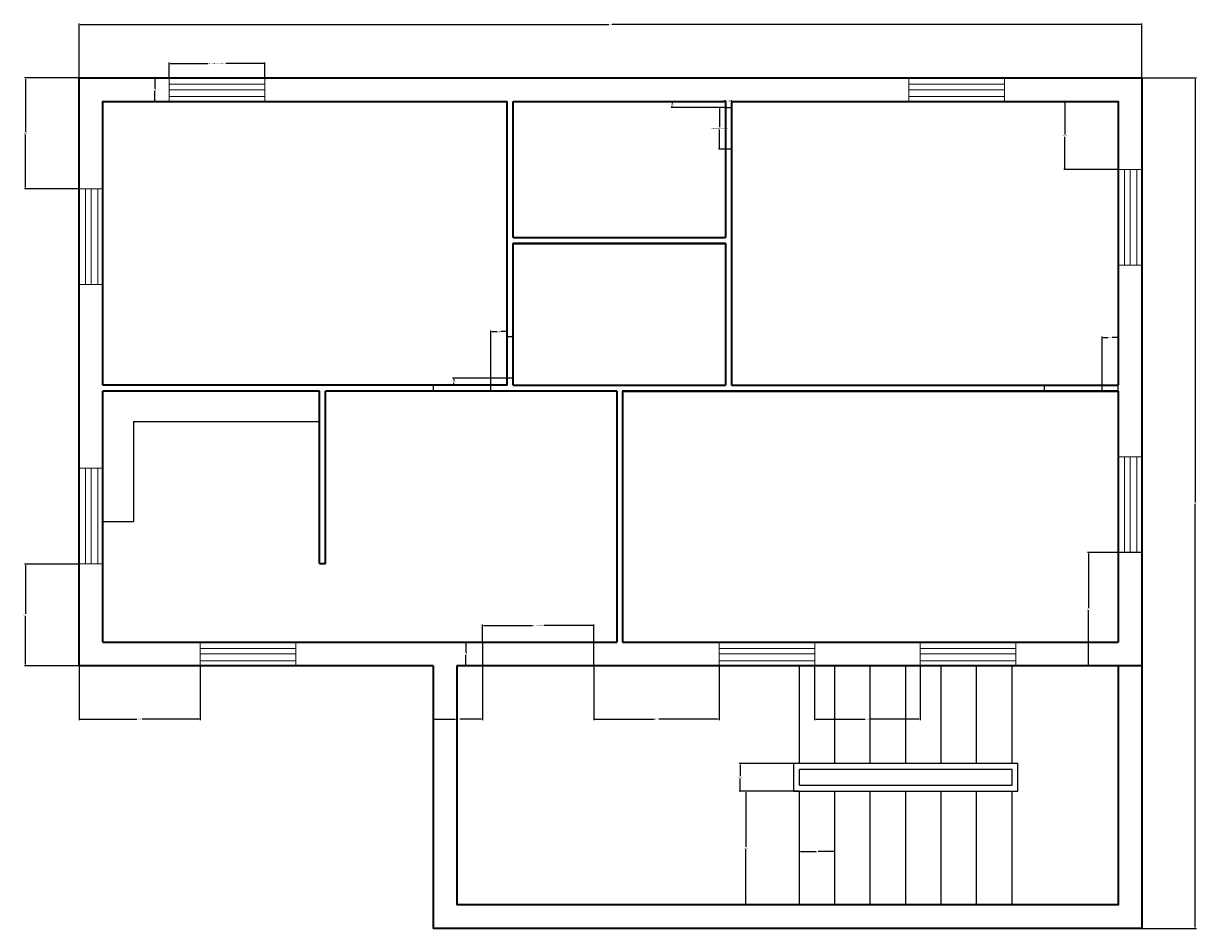
# Model space of a CAD drawing. Units: feet. Extents: x 1914 to 2338, y 2098 to 2528.
# Tile 2 of 3: x 2140 to 2338, y 2107 to 2260. Entities that reach past the tile are written whole.
import ezdxf

# ---------------------------------------------------------------- set-up
doc = ezdxf.new("R2010")
doc.units = ezdxf.units.FT
for name, color, linetype, lineweight in [('A-ANNO-DIMS', 2, 'Continuous', 18), ('A-DOOR', 3, 'Continuous', 25), ('A-FLOR-CASE', 8, 'Continuous', 25), ('A-FLOR-STRS', 7, 'Continuous', 25), ('A-GLAZ', 4, 'Continuous', 18), ('A-WALL', 7, 'Continuous', 35)]:
    doc.layers.add(name, color=color, linetype=linetype, lineweight=lineweight)
doc.styles.get("Standard").update_dxf_attribs({"font": 'arial.ttf'})
doc.dimstyles.get("Standard").update_dxf_attribs({"dimtxt": 0.18, "dimasz": 0.18, "dimexe": 0.18, "dimexo": 0.0625, "dimgap": 0.09, "dimtad": 0, "dimtih": 1, "dimtoh": 1, "dimdec": 1, "dimzin": 0, "dimdsep": 46, "dimlunit": 3, "dimtxsty": 'Standard', "dimcen": 0.09, "dimadec": 0, "dimazin": 0, "dimtfac": 1, "dimtdec": 1, "dimtofl": 0, "dimtmove": 0, "dimatfit": 3, "dimfxl": 1, "dimtolj": 1, "dimtzin": 0, "dimarcsym": 0})

# ---------------------------------------------------------------- blocks, each defined once
blk = doc.blocks.new('WIN-PLAN')
for p, q in [((0, 0), (0, 4)), ((16.2, 4), (16.2, 0)), ((16.2, 2.93), (0, 2.93)), ((16.2, 1.98), (0, 1.98)), ((16.2, 0.84), (0, 0.84))]:
    blk.add_line(p, q)
blk = doc.blocks.new('WIN-PLAN-OUTER-EDGE')
for p, q in [((0, 0), (0, 4)), ((0, 4), (16.2, 4)), ((16.2, 4), (16.2, 0)), ((16.2, 2.93), (0, 2.93)), ((16.2, 1.98), (0, 1.98)), ((16.2, 0.84), (0, 0.84))]:
    blk.add_line(p, q)
blk.add_lwpolyline([(0, 4), (16.2, 4)])
blk = doc.blocks.new('STAIR-RETURN-FLIGHT')
for p, q in [((1, 23.92), (1, 40.5)), ((7, 23.92), (7, 40.5)), ((13, 23.92), (13, 40.5)), ((19, 23.92), (19, 40.5)), ((25, 23.92), (25, 40.5)), ((31, 23.92), (31, 40.5)), ((37, 23.92), (37, 40.5)), ((1, 20.25), (1, 22.92)), ((37, 20.25), (37, 22.92)), ((1, 0), (1, 19.25)), ((7, 0), (7, 19.25)), ((13, 0), (13, 19.25)), ((19, 0), (19, 19.25)), ((25, 0), (25, 19.25)), ((31, 0), (31, 19.25)), ((37, 0), (37, 19.25))]:
    blk.add_line(p, q)
blk.add_lwpolyline([(0, 19.25), (38, 19.25), (38, 23.92), (0, 23.92)], close=True)
for points in [[(37, 22.92), (1, 22.92)], [(1, 20.25), (37, 20.25)]]:
    blk.add_lwpolyline(points)
blk = doc.blocks.new('COUNTER-L')
for p, q in [((5.19, 16.93), (5.19, 0)), ((5.19, 16.93), (36.73, 16.93)), ((0, 0), (5.19, 0))]:
    blk.add_line(p, q)
blk = doc.blocks.new('OPENING-ENTRY')
for points in [[(0, 4), (0, 0)], [(18.83, 0), (18.83, 4)]]:
    blk.add_lwpolyline(points)
blk = doc.blocks.new('OPENING-INTERIOR-WIDE')
blk.add_lwpolyline([(9.8, 0), (9.8, 1), (0, 1), (0, 0)], close=True)
blk = doc.blocks.new('OPENING-INTERIOR-NARROW')
blk.add_lwpolyline([(0, 7.05), (1, 7.05), (1, 0), (0, 0)], close=True)
blk = doc.blocks.new('*D10')
at = {"layer": 'A-ANNO-DIMS', "color": 0, "lineweight": -2, "transparency": 16777216}
for p, q in [((2164.45, 2250.91), (2164.45, 2253.46)), ((2164.63, 2253.28), (2171.05, 2253.28)), ((2180.47, 2253.28), (2174.05, 2253.28)), ((2180.65, 2250.91), (2180.65, 2253.46))]:
    blk.add_line(p, q, dxfattribs=at)
at = {"layer": 'A-ANNO-DIMS', "color": 0, "transparency": 16777216}
for points in [[(2164.63, 2253.31), (2164.63, 2253.25), (2164.45, 2253.28)], [(2180.47, 2253.31), (2180.47, 2253.25), (2180.65, 2253.28)]]:
    blk.add_solid(points, dxfattribs=at)
at = {"layer": 'Defpoints', "color": 0, "transparency": 16777216}
for p in [(2180.65, 2253.28), (2164.45, 2250.85), (2180.65, 2250.85)]:
    blk.add_point(p, dxfattribs=at)
at = {"layer": 'A-ANNO-DIMS', "color": 0, "transparency": 16777216, "insert": (2172.55, 2253.28), "char_height": 0.18, "attachment_point": 5}
blk.add_mtext('\\A1;EDGE WINDOW 16 TYP.', dxfattribs=at)
blk = doc.blocks.new('*D11')
at = {"layer": 'A-ANNO-DIMS', "color": 0, "lineweight": -2, "transparency": 16777216}
for p, q in [((2164.39, 2250.85), (2161.84, 2250.85)), ((2162.02, 2250.67), (2162.02, 2249.03)), ((2162.02, 2247.03), (2162.02, 2248.67)), ((2164.39, 2246.85), (2161.84, 2246.85))]:
    blk.add_line(p, q, dxfattribs=at)
at = {"layer": 'A-ANNO-DIMS', "color": 0, "transparency": 16777216}
for points in [[(2161.99, 2250.67), (2162.05, 2250.67), (2162.02, 2250.85)], [(2161.99, 2247.03), (2162.05, 2247.03), (2162.02, 2246.85)]]:
    blk.add_solid(points, dxfattribs=at)
at = {"layer": 'Defpoints', "color": 0, "transparency": 16777216}
for p in [(2162.02, 2250.85), (2164.45, 2250.85), (2164.45, 2246.85)]:
    blk.add_point(p, dxfattribs=at)
at = {"layer": 'A-ANNO-DIMS', "color": 0, "transparency": 16777216, "insert": (2162.02, 2248.85), "char_height": 0.18, "attachment_point": 5}
blk.add_mtext('\\A1;4 TYP.', dxfattribs=at)
blk = doc.blocks.new('*D14')
at = {"layer": 'A-ANNO-DIMS', "color": 0, "lineweight": -2, "transparency": 16777216}
for p, q in [((2258.63, 2245.84), (2257.46, 2245.84)), ((2257.64, 2245.66), (2257.64, 2242.5)), ((2257.64, 2238.97), (2257.64, 2242.13)), ((2258.63, 2238.79), (2257.46, 2238.79))]:
    blk.add_line(p, q, dxfattribs=at)
at = {"layer": 'A-ANNO-DIMS', "color": 0, "transparency": 16777216}
for points in [[(2257.61, 2245.66), (2257.67, 2245.66), (2257.64, 2245.84)], [(2257.61, 2238.97), (2257.67, 2238.97), (2257.64, 2238.79)]]:
    blk.add_solid(points, dxfattribs=at)
at = {"layer": 'Defpoints', "color": 0, "transparency": 16777216}
for p in [(2257.64, 2245.84), (2258.69, 2245.84), (2258.69, 2238.79)]:
    blk.add_point(p, dxfattribs=at)
at = {"layer": 'A-ANNO-DIMS', "color": 0, "transparency": 16777216, "insert": (2257.64, 2242.31), "char_height": 0.18, "attachment_point": 5}
blk.add_mtext('\\A1;NARROW OPENING 7 TYP.', dxfattribs=at)
blk = doc.blocks.new('*D15')
at = {"layer": 'A-ANNO-DIMS', "color": 0, "lineweight": -2, "transparency": 16777216}
for p, q in [((2258.69, 2245.9), (2258.69, 2247.08)), ((2259.69, 2245.9), (2259.69, 2247.08)), ((2258.51, 2246.9), (2258.33, 2246.9)), ((2259.87, 2246.9), (2260.05, 2246.9))]:
    blk.add_line(p, q, dxfattribs=at)
at = {"layer": 'A-ANNO-DIMS', "color": 0, "transparency": 16777216}
for points in [[(2258.51, 2246.93), (2258.51, 2246.87), (2258.69, 2246.9)], [(2259.87, 2246.93), (2259.87, 2246.87), (2259.69, 2246.9)]]:
    blk.add_solid(points, dxfattribs=at)
at = {"layer": 'Defpoints', "color": 0, "transparency": 16777216}
for p in [(2258.69, 2245.84), (2259.69, 2246.9), (2259.69, 2245.84)]:
    blk.add_point(p, dxfattribs=at)
at = {"layer": 'A-ANNO-DIMS', "color": 0, "transparency": 16777216, "insert": (2259.19, 2246.9), "char_height": 0.18, "attachment_point": 5}
blk.add_mtext('\\A1;1 TYP.', dxfattribs=at)
blk = doc.blocks.new('*D16')
at = {"layer": 'A-ANNO-DIMS', "color": 0, "lineweight": -2, "transparency": 16777216}
for p, q in [((2217.53, 2155.41), (2217.53, 2158.35)), ((2217.71, 2158.17), (2225.96, 2158.17)), ((2236.18, 2158.17), (2227.93, 2158.17)), ((2236.36, 2155.41), (2236.36, 2158.35))]:
    blk.add_line(p, q, dxfattribs=at)
at = {"layer": 'A-ANNO-DIMS', "color": 0, "transparency": 16777216}
for points in [[(2217.71, 2158.2), (2217.71, 2158.14), (2217.53, 2158.17)], [(2236.18, 2158.2), (2236.18, 2158.14), (2236.36, 2158.17)]]:
    blk.add_solid(points, dxfattribs=at)
at = {"layer": 'Defpoints', "color": 0, "transparency": 16777216}
for p in [(2236.36, 2158.17), (2217.53, 2155.35), (2236.36, 2155.35)]:
    blk.add_point(p, dxfattribs=at)
at = {"layer": 'A-ANNO-DIMS', "color": 0, "transparency": 16777216, "insert": (2226.94, 2158.17), "char_height": 0.18, "attachment_point": 5}
blk.add_mtext('\\A1;ENTRY 19 TYP.', dxfattribs=at)
blk = doc.blocks.new('*D17')
at = {"layer": 'A-ANNO-DIMS', "color": 0, "lineweight": -2, "transparency": 16777216}
for p, q in [((2217.46, 2155.35), (2214.52, 2155.35)), ((2214.7, 2155.17), (2214.7, 2153.53)), ((2214.7, 2151.53), (2214.7, 2153.17)), ((2217.46, 2151.35), (2214.52, 2151.35))]:
    blk.add_line(p, q, dxfattribs=at)
at = {"layer": 'A-ANNO-DIMS', "color": 0, "transparency": 16777216}
for points in [[(2214.67, 2155.17), (2214.73, 2155.17), (2214.7, 2155.35)], [(2214.67, 2151.53), (2214.73, 2151.53), (2214.7, 2151.35)]]:
    blk.add_solid(points, dxfattribs=at)
at = {"layer": 'Defpoints', "color": 0, "transparency": 16777216}
for p in [(2214.7, 2155.35), (2217.53, 2155.35), (2217.53, 2151.35)]:
    blk.add_point(p, dxfattribs=at)
at = {"layer": 'A-ANNO-DIMS', "color": 0, "transparency": 16777216, "insert": (2214.7, 2153.35), "char_height": 0.18, "attachment_point": 5}
blk.add_mtext('\\A1;4 TYP.', dxfattribs=at)
blk = doc.blocks.new('*D35')
at = {"layer": 'A-ANNO-DIMS', "color": 0, "lineweight": -2, "transparency": 16777216}
for p, q in [((2271.19, 2110.91), (2271.19, 2120.08)), ((2277.19, 2110.91), (2277.19, 2120.08)), ((2271.37, 2119.9), (2274.04, 2119.9)), ((2277.01, 2119.9), (2274.34, 2119.9))]:
    blk.add_line(p, q, dxfattribs=at)
at = {"layer": 'A-ANNO-DIMS', "color": 0, "transparency": 16777216}
for points in [[(2271.37, 2119.93), (2271.37, 2119.87), (2271.19, 2119.9)], [(2277.01, 2119.93), (2277.01, 2119.87), (2277.19, 2119.9)]]:
    blk.add_solid(points, dxfattribs=at)
at = {"layer": 'Defpoints', "color": 0, "transparency": 16777216}
for p in [(2277.19, 2119.9), (2271.19, 2110.85), (2277.19, 2110.85)]:
    blk.add_point(p, dxfattribs=at)
at = {"layer": 'A-ANNO-DIMS', "color": 0, "transparency": 16777216, "insert": (2274.19, 2119.9), "char_height": 0.18, "attachment_point": 5}
blk.add_mtext('\\A1;6', dxfattribs=at)
blk = doc.blocks.new('*D36')
at = {"layer": 'A-ANNO-DIMS', "color": 0, "lineweight": -2, "transparency": 16777216}
for p, q in [((2271.13, 2130.1), (2261.96, 2130.1)), ((2262.14, 2129.92), (2262.14, 2120.66)), ((2262.14, 2111.03), (2262.14, 2120.29)), ((2271.13, 2110.85), (2261.96, 2110.85))]:
    blk.add_line(p, q, dxfattribs=at)
at = {"layer": 'A-ANNO-DIMS', "color": 0, "transparency": 16777216}
for points in [[(2262.11, 2129.92), (2262.17, 2129.92), (2262.14, 2130.1)], [(2262.11, 2111.03), (2262.17, 2111.03), (2262.14, 2110.85)]]:
    blk.add_solid(points, dxfattribs=at)
at = {"layer": 'Defpoints', "color": 0, "transparency": 16777216}
for p in [(2262.14, 2130.1), (2271.19, 2130.1), (2271.19, 2110.85)]:
    blk.add_point(p, dxfattribs=at)
at = {"layer": 'A-ANNO-DIMS', "color": 0, "transparency": 16777216, "insert": (2262.14, 2120.47), "char_height": 0.18, "attachment_point": 5}
blk.add_mtext('\\A1;19.25', dxfattribs=at)
blk = doc.blocks.new('*D37')
at = {"layer": 'A-ANNO-DIMS', "color": 0, "lineweight": -2, "transparency": 16777216}
for p, q in [((2270.13, 2134.77), (2260.96, 2134.77)), ((2261.14, 2134.59), (2261.14, 2132.62)), ((2261.14, 2130.28), (2261.14, 2132.25)), ((2270.13, 2130.1), (2260.96, 2130.1))]:
    blk.add_line(p, q, dxfattribs=at)
at = {"layer": 'A-ANNO-DIMS', "color": 0, "transparency": 16777216}
for points in [[(2261.11, 2134.59), (2261.17, 2134.59), (2261.14, 2134.77)], [(2261.11, 2130.28), (2261.17, 2130.28), (2261.14, 2130.1)]]:
    blk.add_solid(points, dxfattribs=at)
at = {"layer": 'Defpoints', "color": 0, "transparency": 16777216}
for p in [(2261.14, 2134.77), (2270.19, 2134.77), (2270.19, 2130.1)]:
    blk.add_point(p, dxfattribs=at)
at = {"layer": 'A-ANNO-DIMS', "color": 0, "transparency": 16777216, "insert": (2261.14, 2132.43), "char_height": 0.18, "attachment_point": 5}
blk.add_mtext('\\A1;4.671', dxfattribs=at)
blk = doc.blocks.new('*D38')
at = {"layer": 'A-ANNO-DIMS', "color": 0, "lineweight": -2, "transparency": 16777216}
for p, q in [((2149.19, 2250.91), (2149.19, 2260.08)), ((2149.37, 2259.9), (2238.91, 2259.9)), ((2329.01, 2259.9), (2239.47, 2259.9)), ((2329.19, 2250.91), (2329.19, 2260.08))]:
    blk.add_line(p, q, dxfattribs=at)
at = {"layer": 'A-ANNO-DIMS', "color": 0, "transparency": 16777216}
for points in [[(2149.37, 2259.93), (2149.37, 2259.87), (2149.19, 2259.9)], [(2329.01, 2259.93), (2329.01, 2259.87), (2329.19, 2259.9)]]:
    blk.add_solid(points, dxfattribs=at)
at = {"layer": 'Defpoints', "color": 0, "transparency": 16777216}
for p in [(2329.19, 2259.9), (2149.19, 2250.85), (2329.19, 2250.85)]:
    blk.add_point(p, dxfattribs=at)
at = {"layer": 'A-ANNO-DIMS', "color": 0, "transparency": 16777216, "insert": (2239.19, 2259.9), "char_height": 0.18, "attachment_point": 5}
blk.add_mtext('\\A1;180', dxfattribs=at)
blk = doc.blocks.new('*D39')
at = {"layer": 'A-ANNO-DIMS', "color": 0, "lineweight": -2, "transparency": 16777216}
for p, q in [((2329.26, 2250.85), (2338.42, 2250.85)), ((2338.24, 2250.67), (2338.24, 2179.03)), ((2338.24, 2107.03), (2338.24, 2178.67)), ((2329.26, 2106.85), (2338.42, 2106.85))]:
    blk.add_line(p, q, dxfattribs=at)
at = {"layer": 'A-ANNO-DIMS', "color": 0, "transparency": 16777216}
for points in [[(2338.21, 2250.67), (2338.27, 2250.67), (2338.24, 2250.85)], [(2338.21, 2107.03), (2338.27, 2107.03), (2338.24, 2106.85)]]:
    blk.add_solid(points, dxfattribs=at)
at = {"layer": 'Defpoints', "color": 0, "transparency": 16777216}
for p in [(2329.19, 2250.85), (2338.24, 2250.85), (2329.19, 2106.85)]:
    blk.add_point(p, dxfattribs=at)
at = {"layer": 'A-ANNO-DIMS', "color": 0, "transparency": 16777216, "insert": (2338.24, 2178.85), "char_height": 0.18, "attachment_point": 5}
blk.add_mtext('\\A1;144', dxfattribs=at)
blk = doc.blocks.new('*D42')
at = {"layer": 'A-ANNO-DIMS', "color": 0, "lineweight": -2, "transparency": 16777216}
for p, q in [((2149.13, 2250.85), (2139.96, 2250.85)), ((2140.14, 2250.67), (2140.14, 2241.66)), ((2140.14, 2232.28), (2140.14, 2241.29)), ((2149.13, 2232.1), (2139.96, 2232.1))]:
    blk.add_line(p, q, dxfattribs=at)
at = {"layer": 'A-ANNO-DIMS', "color": 0, "transparency": 16777216}
for points in [[(2140.11, 2250.67), (2140.17, 2250.67), (2140.14, 2250.85)], [(2140.11, 2232.28), (2140.17, 2232.28), (2140.14, 2232.1)]]:
    blk.add_solid(points, dxfattribs=at)
at = {"layer": 'Defpoints', "color": 0, "transparency": 16777216}
for p in [(2140.14, 2250.85), (2149.19, 2250.85), (2149.19, 2232.1)]:
    blk.add_point(p, dxfattribs=at)
at = {"layer": 'A-ANNO-DIMS', "color": 0, "transparency": 16777216, "insert": (2140.14, 2241.47), "char_height": 0.18, "attachment_point": 5}
blk.add_mtext('\\A1;18.75', dxfattribs=at)
blk = doc.blocks.new('*D43')
at = {"layer": 'A-ANNO-DIMS', "color": 0, "lineweight": -2, "transparency": 16777216}
for p, q in [((2149.13, 2168.56), (2139.96, 2168.56)), ((2140.14, 2168.38), (2140.14, 2160.14)), ((2140.14, 2151.53), (2140.14, 2159.77)), ((2149.13, 2151.35), (2139.96, 2151.35))]:
    blk.add_line(p, q, dxfattribs=at)
at = {"layer": 'A-ANNO-DIMS', "color": 0, "transparency": 16777216}
for points in [[(2140.11, 2168.38), (2140.17, 2168.38), (2140.14, 2168.56)], [(2140.11, 2151.53), (2140.17, 2151.53), (2140.14, 2151.35)]]:
    blk.add_solid(points, dxfattribs=at)
at = {"layer": 'Defpoints', "color": 0, "transparency": 16777216}
for p in [(2140.14, 2168.56), (2149.19, 2168.56), (2149.19, 2151.35)]:
    blk.add_point(p, dxfattribs=at)
at = {"layer": 'A-ANNO-DIMS', "color": 0, "transparency": 16777216, "insert": (2140.14, 2159.96), "char_height": 0.18, "attachment_point": 5}
blk.add_mtext('\\A1;17.216', dxfattribs=at)
blk = doc.blocks.new('*D44')
at = {"layer": 'A-ANNO-DIMS', "color": 0, "lineweight": -2, "transparency": 16777216}
for p, q in [((2325.13, 2246.85), (2315.96, 2246.85)), ((2316.14, 2246.67), (2316.14, 2241.28)), ((2316.14, 2235.52), (2316.14, 2240.91)), ((2325.13, 2235.34), (2315.96, 2235.34))]:
    blk.add_line(p, q, dxfattribs=at)
at = {"layer": 'A-ANNO-DIMS', "color": 0, "transparency": 16777216}
for points in [[(2316.11, 2246.67), (2316.17, 2246.67), (2316.14, 2246.85)], [(2316.11, 2235.52), (2316.17, 2235.52), (2316.14, 2235.34)]]:
    blk.add_solid(points, dxfattribs=at)
at = {"layer": 'Defpoints', "color": 0, "transparency": 16777216}
for p in [(2316.14, 2246.85), (2325.19, 2246.85), (2325.19, 2235.34)]:
    blk.add_point(p, dxfattribs=at)
at = {"layer": 'A-ANNO-DIMS', "color": 0, "transparency": 16777216, "insert": (2316.14, 2241.1), "char_height": 0.18, "attachment_point": 5}
blk.add_mtext('\\A1;11.505', dxfattribs=at)
blk = doc.blocks.new('*D45')
at = {"layer": 'A-ANNO-DIMS', "color": 0, "lineweight": -2, "transparency": 16777216}
for p, q in [((2329.13, 2170.51), (2319.96, 2170.51)), ((2320.14, 2170.33), (2320.14, 2161.11)), ((2320.14, 2151.53), (2320.14, 2160.75)), ((2329.13, 2151.35), (2319.96, 2151.35))]:
    blk.add_line(p, q, dxfattribs=at)
at = {"layer": 'A-ANNO-DIMS', "color": 0, "transparency": 16777216}
for points in [[(2320.11, 2170.33), (2320.17, 2170.33), (2320.14, 2170.51)], [(2320.11, 2151.53), (2320.17, 2151.53), (2320.14, 2151.35)]]:
    blk.add_solid(points, dxfattribs=at)
at = {"layer": 'Defpoints', "color": 0, "transparency": 16777216}
for p in [(2320.14, 2170.51), (2329.19, 2170.51), (2329.19, 2151.35)]:
    blk.add_point(p, dxfattribs=at)
at = {"layer": 'A-ANNO-DIMS', "color": 0, "transparency": 16777216, "insert": (2320.14, 2160.93), "char_height": 0.18, "attachment_point": 5}
blk.add_mtext('\\A1;19.165', dxfattribs=at)
blk = doc.blocks.new('*D46')
at = {"layer": 'A-ANNO-DIMS', "color": 0, "lineweight": -2, "transparency": 16777216}
for p, q in [((2149.19, 2151.29), (2149.19, 2142.12)), ((2169.68, 2151.29), (2169.68, 2142.12)), ((2149.37, 2142.3), (2158.97, 2142.3)), ((2169.5, 2142.3), (2159.9, 2142.3))]:
    blk.add_line(p, q, dxfattribs=at)
at = {"layer": 'A-ANNO-DIMS', "color": 0, "transparency": 16777216}
for points in [[(2149.37, 2142.33), (2149.37, 2142.27), (2149.19, 2142.3)], [(2169.5, 2142.33), (2169.5, 2142.27), (2169.68, 2142.3)]]:
    blk.add_solid(points, dxfattribs=at)
at = {"layer": 'Defpoints', "color": 0, "transparency": 16777216}
for p in [(2149.19, 2151.35), (2169.68, 2151.35), (2149.19, 2142.3)]:
    blk.add_point(p, dxfattribs=at)
at = {"layer": 'A-ANNO-DIMS', "color": 0, "transparency": 16777216, "insert": (2159.44, 2142.3), "char_height": 0.18, "attachment_point": 5}
blk.add_mtext('\\A1;20.486', dxfattribs=at)
blk = doc.blocks.new('*D47')
at = {"layer": 'A-ANNO-DIMS', "color": 0, "lineweight": -2, "transparency": 16777216}
for p, q in [((2209.18, 2151.29), (2209.18, 2142.12)), ((2217.53, 2151.29), (2217.53, 2142.12)), ((2209.36, 2142.3), (2212.96, 2142.3)), ((2217.35, 2142.3), (2213.75, 2142.3))]:
    blk.add_line(p, q, dxfattribs=at)
at = {"layer": 'A-ANNO-DIMS', "color": 0, "transparency": 16777216}
for points in [[(2209.36, 2142.33), (2209.36, 2142.27), (2209.18, 2142.3)], [(2217.35, 2142.33), (2217.35, 2142.27), (2217.53, 2142.3)]]:
    blk.add_solid(points, dxfattribs=at)
at = {"layer": 'Defpoints', "color": 0, "transparency": 16777216}
for p in [(2209.18, 2151.35), (2217.53, 2151.35), (2209.18, 2142.3)]:
    blk.add_point(p, dxfattribs=at)
at = {"layer": 'A-ANNO-DIMS', "color": 0, "transparency": 16777216, "insert": (2213.35, 2142.3), "char_height": 0.18, "attachment_point": 5}
blk.add_mtext('\\A1;8.349', dxfattribs=at)
blk = doc.blocks.new('*D48')
at = {"layer": 'A-ANNO-DIMS', "color": 0, "lineweight": -2, "transparency": 16777216}
for p, q in [((2236.36, 2151.29), (2236.36, 2142.12)), ((2257.58, 2151.29), (2257.58, 2142.12)), ((2236.54, 2142.3), (2246.57, 2142.3)), ((2257.4, 2142.3), (2247.36, 2142.3))]:
    blk.add_line(p, q, dxfattribs=at)
at = {"layer": 'A-ANNO-DIMS', "color": 0, "transparency": 16777216}
for points in [[(2236.54, 2142.33), (2236.54, 2142.27), (2236.36, 2142.3)], [(2257.4, 2142.33), (2257.4, 2142.27), (2257.58, 2142.3)]]:
    blk.add_solid(points, dxfattribs=at)
at = {"layer": 'Defpoints', "color": 0, "transparency": 16777216}
for p in [(2236.36, 2151.35), (2257.58, 2151.35), (2236.36, 2142.3)]:
    blk.add_point(p, dxfattribs=at)
at = {"layer": 'A-ANNO-DIMS', "color": 0, "transparency": 16777216, "insert": (2246.97, 2142.3), "char_height": 0.18, "attachment_point": 5}
blk.add_mtext('\\A1;21.22', dxfattribs=at)
blk = doc.blocks.new('*D49')
at = {"layer": 'A-ANNO-DIMS', "color": 0, "lineweight": -2, "transparency": 16777216}
for p, q in [((2273.77, 2151.29), (2273.77, 2142.12)), ((2291.62, 2151.29), (2291.62, 2142.12)), ((2273.95, 2142.3), (2282.31, 2142.3)), ((2291.44, 2142.3), (2283.08, 2142.3))]:
    blk.add_line(p, q, dxfattribs=at)
at = {"layer": 'A-ANNO-DIMS', "color": 0, "transparency": 16777216}
for points in [[(2273.95, 2142.33), (2273.95, 2142.27), (2273.77, 2142.3)], [(2291.44, 2142.33), (2291.44, 2142.27), (2291.62, 2142.3)]]:
    blk.add_solid(points, dxfattribs=at)
at = {"layer": 'Defpoints', "color": 0, "transparency": 16777216}
for p in [(2273.77, 2151.35), (2291.62, 2151.35), (2273.77, 2142.3)]:
    blk.add_point(p, dxfattribs=at)
at = {"layer": 'A-ANNO-DIMS', "color": 0, "transparency": 16777216, "insert": (2282.7, 2142.3), "char_height": 0.18, "attachment_point": 5}
blk.add_mtext('\\A1;17.85', dxfattribs=at)
blk = doc.blocks.new('*D50')
at = {"layer": 'A-ANNO-DIMS', "color": 0, "lineweight": -2, "transparency": 16777216}
for p, q in [((2218.94, 2198.91), (2218.94, 2208.08)), ((2219.12, 2207.9), (2219.99, 2207.9)), ((2221.51, 2207.9), (2220.64, 2207.9)), ((2221.69, 2198.91), (2221.69, 2208.08))]:
    blk.add_line(p, q, dxfattribs=at)
at = {"layer": 'A-ANNO-DIMS', "color": 0, "transparency": 16777216}
for points in [[(2219.12, 2207.93), (2219.12, 2207.87), (2218.94, 2207.9)], [(2221.51, 2207.93), (2221.51, 2207.87), (2221.69, 2207.9)]]:
    blk.add_solid(points, dxfattribs=at)
at = {"layer": 'Defpoints', "color": 0, "transparency": 16777216}
for p in [(2221.69, 2207.9), (2218.94, 2198.85), (2221.69, 2198.85)]:
    blk.add_point(p, dxfattribs=at)
at = {"layer": 'A-ANNO-DIMS', "color": 0, "transparency": 16777216, "insert": (2220.31, 2207.9), "char_height": 0.18, "attachment_point": 5}
blk.add_mtext('\\A1;2.76', dxfattribs=at)
blk = doc.blocks.new('*D51')
at = {"layer": 'A-ANNO-DIMS', "color": 0, "lineweight": -2, "transparency": 16777216}
for p, q in [((2322.44, 2197.91), (2322.44, 2207.08)), ((2322.62, 2206.9), (2323.49, 2206.9)), ((2325.01, 2206.9), (2324.14, 2206.9)), ((2325.19, 2197.91), (2325.19, 2207.08))]:
    blk.add_line(p, q, dxfattribs=at)
at = {"layer": 'A-ANNO-DIMS', "color": 0, "transparency": 16777216}
for points in [[(2322.62, 2206.93), (2322.62, 2206.87), (2322.44, 2206.9)], [(2325.01, 2206.93), (2325.01, 2206.87), (2325.19, 2206.9)]]:
    blk.add_solid(points, dxfattribs=at)
at = {"layer": 'Defpoints', "color": 0, "transparency": 16777216}
for p in [(2325.19, 2206.9), (2322.44, 2197.85), (2325.19, 2197.85)]:
    blk.add_point(p, dxfattribs=at)
at = {"layer": 'A-ANNO-DIMS', "color": 0, "transparency": 16777216, "insert": (2323.81, 2206.9), "char_height": 0.18, "attachment_point": 5}
blk.add_mtext('\\A1;2.76', dxfattribs=at)
blk = doc.blocks.new('*D52')
at = {"layer": 'A-ANNO-DIMS', "color": 0, "lineweight": -2, "transparency": 16777216}
for p, q in [((2221.63, 2200.03), (2212.46, 2200.03)), ((2212.64, 2199.85), (2212.64, 2199.62)), ((2221.63, 2198.85), (2212.46, 2198.85)), ((2212.64, 2199.03), (2212.64, 2199.26))]:
    blk.add_line(p, q, dxfattribs=at)
at = {"layer": 'A-ANNO-DIMS', "color": 0, "transparency": 16777216}
for points in [[(2212.61, 2199.85), (2212.67, 2199.85), (2212.64, 2200.03)], [(2212.61, 2199.03), (2212.67, 2199.03), (2212.64, 2198.85)]]:
    blk.add_solid(points, dxfattribs=at)
at = {"layer": 'Defpoints', "color": 0, "transparency": 16777216}
for p in [(2212.64, 2200.03), (2221.69, 2200.03), (2221.69, 2198.85)]:
    blk.add_point(p, dxfattribs=at)
at = {"layer": 'A-ANNO-DIMS', "color": 0, "transparency": 16777216, "insert": (2212.64, 2199.44), "char_height": 0.18, "attachment_point": 5}
blk.add_mtext('\\A1;1.179', dxfattribs=at)
blk = doc.blocks.new('*D53')
at = {"layer": 'A-ANNO-DIMS', "color": 0, "lineweight": -2, "transparency": 16777216}
for p, q in [((2258.63, 2246.85), (2249.46, 2246.85)), ((2258.63, 2245.84), (2249.46, 2245.84)), ((2249.64, 2246.67), (2249.64, 2246.53)), ((2249.64, 2246.02), (2249.64, 2246.16))]:
    blk.add_line(p, q, dxfattribs=at)
at = {"layer": 'A-ANNO-DIMS', "color": 0, "transparency": 16777216}
for points in [[(2249.61, 2246.67), (2249.67, 2246.67), (2249.64, 2246.85)], [(2249.61, 2246.02), (2249.67, 2246.02), (2249.64, 2245.84)]]:
    blk.add_solid(points, dxfattribs=at)
at = {"layer": 'Defpoints', "color": 0, "transparency": 16777216}
for p in [(2249.64, 2246.85), (2258.69, 2246.85), (2258.69, 2245.84)]:
    blk.add_point(p, dxfattribs=at)
at = {"layer": 'A-ANNO-DIMS', "color": 0, "transparency": 16777216, "insert": (2249.64, 2246.34), "char_height": 0.18, "attachment_point": 5}
blk.add_mtext('\\A1;1.01', dxfattribs=at)

msp = doc.modelspace()

# ---------------------------------------------------------------- linework, layer by layer
at = {"layer": 'A-WALL'}
for p, q in [((2240.2478, 2197.8486), (2222.3605, 2197.8486)), ((2222.6937, 2198.8486), (2258.6937, 2198.8486)), ((2240.2478, 2197.8486), (2240.2478, 2155.3486)), ((2241.1937, 2197.8486), (2325.1937, 2197.8486)), ((2325.1937, 2197.8486), (2241.2478, 2197.8486)), ((2241.2478, 2197.8486), (2241.2478, 2155.3486)), ((2259.6937, 2198.8486), (2325.1937, 2198.8486)), ((2189.9261, 2168.6719), (2190.9261, 2168.6719)), ((2213.1769, 2155.3486), (2240.2478, 2155.3486)), ((2241.2478, 2155.3486), (2325.1937, 2155.3486)), ((2325.1937, 2151.3486), (2313.1937, 2151.3486)), ((2209.1769, 2110.8486), (2209.1769, 2106.8486))]:
    msp.add_line(p, q, dxfattribs=at)
for points in [[(2149.1937, 2151.3486), (2149.1937, 2250.8486), (2329.1937, 2250.8486), (2329.1937, 2106.8486), (2209.1769, 2106.8486)], [(2153.1937, 2198.8486), (2153.1937, 2246.8486), (2221.6937, 2246.8486)], [(2221.6937, 2198.8486), (2221.6937, 2246.8486)], [(2222.6937, 2246.8486), (2258.6937, 2246.8486)], [(2222.6937, 2223.8486), (2222.6937, 2246.8486)], [(2258.6937, 2246.8486), (2258.6937, 2223.8486)], [(2259.6937, 2246.8486), (2325.1937, 2246.8486), (2325.1937, 2198.8486)], [(2259.6937, 2246.8486), (2259.6937, 2198.8486)], [(2222.6937, 2223.8486), (2258.6937, 2223.8486)], [(2258.6937, 2222.8486), (2222.6937, 2222.8486)], [(2222.6937, 2198.8486), (2222.6937, 2222.8486), (2258.6937, 2222.8486), (2258.6937, 2198.8486)], [(2221.6937, 2198.8486), (2153.1937, 2198.8486)], [(2153.1937, 2155.3486), (2153.1937, 2197.8486)], [(2189.9261, 2197.8486), (2153.1937, 2197.8486)], [(2189.9261, 2168.6719), (2189.9261, 2197.8486)], [(2240.2478, 2197.8486), (2190.9261, 2197.8486)], [(2190.9261, 2168.6719), (2190.9261, 2197.8486)], [(2325.1937, 2197.8486), (2325.1937, 2155.3486)], [(2153.1937, 2155.3486), (2213.1769, 2155.3486)], [(2209.1769, 2151.3486), (2149.1937, 2151.3486)], [(2209.1769, 2151.3486), (2209.1769, 2110.8486)], [(2325.1937, 2151.3486), (2325.1937, 2110.8486), (2213.1769, 2110.8486)], [(2213.1769, 2151.3486), (2213.1769, 2110.8486)], [(2329.1937, 2151.3486), (2213.1769, 2151.3486)]]:
    msp.add_lwpolyline(points, dxfattribs=at)

# ---------------------------------------------------------------- block references
at = {"layer": 'A-DOOR'}
for name, p in [('OPENING-INTERIOR-NARROW', (2258.6937, 2238.7895)), ('OPENING-INTERIOR-NARROW', (2221.6937, 2200.0275)), ('OPENING-INTERIOR-WIDE', (2209.1371, 2197.8486)), ('OPENING-INTERIOR-WIDE', (2312.6371, 2197.8486)), ('OPENING-ENTRY', (2217.5254, 2151.3486))]:
    msp.add_blockref(name, p, dxfattribs=at)
at = {"layer": 'A-FLOR-CASE'}
msp.add_blockref('COUNTER-L', (2153.1937, 2175.7782), dxfattribs=at)
at = {"layer": 'A-FLOR-STRS'}
msp.add_blockref('STAIR-RETURN-FLIGHT', (2270.1937, 2110.8486), dxfattribs=at)
at = {"layer": 'A-GLAZ'}
for name, p in [('WIN-PLAN-OUTER-EDGE', (2164.4517, 2246.8486)), ('WIN-PLAN', (2289.7022, 2246.8486)), ('WIN-PLAN', (2169.68, 2151.3486)), ('WIN-PLAN', (2257.5751, 2151.3486)), ('WIN-PLAN', (2291.6233, 2151.3486))]:
    msp.add_blockref(name, p, dxfattribs=at)
for p, rotation in [((2329.1937, 2219.144), 90.00000000000378), ((2153.1937, 2215.9), 90.00000000000378), ((2329.1937, 2170.5134), 90.00000000000453), ((2153.1937, 2168.565), 90.00000000000453)]:
    msp.add_blockref('WIN-PLAN', p, dxfattribs=dict(at, rotation=rotation))

# ---------------------------------------------------------------- dimensions: what is measured, and where the dimension line sits
at = {"layer": 'A-ANNO-DIMS'}
for base, p1, p2, override, picture, middle in [((2329.1937, 2259.8986), (2149.1937, 2250.8486), (2329.1937, 2250.8486), {"dimdec": 0, "dimlfac": 1, "dimrnd": 0, "dimzin": 0, "dimdsep": 46, "dimlunit": 2}, '*D38', (2239.1937, 2259.8986)), ((2325.1937, 2206.8986), (2322.4355, 2197.8486), (2325.1937, 2197.8486), {"dimdec": 2, "dimlfac": 1, "dimrnd": 0, "dimzin": 0, "dimdsep": 46, "dimlunit": 2}, '*D51', (2323.8146, 2206.8986)), ((2277.1937, 2119.8986), (2271.1937, 2110.8486), (2277.1937, 2110.8486), {"dimdec": 0, "dimlfac": 1, "dimrnd": 0, "dimzin": 0, "dimdsep": 46, "dimlunit": 2}, '*D35', (2274.1937, 2119.8986))]:
    dim = msp.add_linear_dim(base=base, p1=p1, p2=p2, dimstyle='Standard', override=override, dxfattribs=at)
    dim.commit()
    dim.dimension.update_dxf_attribs({"geometry": picture, "text_midpoint": middle})
for base, p1, p2, text, picture, middle in [((2180.6509, 2253.2785), (2164.4517, 2250.8486), (2180.6509, 2250.8486), 'EDGE WINDOW <> TYP.', '*D10', (2172.5513, 2253.2785)), ((2259.6937, 2246.8957), (2258.6937, 2245.8384), (2259.6937, 2245.8384), '<> TYP.', '*D15', (2259.1937, 2246.8957)), ((2236.3564, 2158.1732), (2217.5254, 2155.3486), (2236.3564, 2155.3486), 'ENTRY <> TYP.', '*D16', (2226.9409, 2158.1732))]:
    dim = msp.add_linear_dim(base=base, p1=p1, p2=p2, text=text, dimstyle='Standard', override={"dimdec": 0, "dimlfac": 1, "dimrnd": 0, "dimzin": 0, "dimdsep": 46, "dimlunit": 2}, dxfattribs=at)
    dim.commit()
    dim.dimension.update_dxf_attribs({"geometry": picture, "text_midpoint": middle})
for base, p1, p2, angle, override, picture, middle in [((2140.1437, 2250.8486), (2149.1937, 2232.0992), (2149.1937, 2250.8486), 90, {"dimdec": 2, "dimlfac": 1, "dimrnd": 0, "dimzin": 0, "dimdsep": 46, "dimlunit": 2}, '*D42', (2140.1437, 2241.4739)), ((2338.2437, 2250.8486), (2329.1937, 2106.8486), (2329.1937, 2250.8486), 90, {"dimdec": 0, "dimlfac": 1, "dimrnd": 0, "dimzin": 0, "dimdsep": 46, "dimlunit": 2}, '*D39', (2338.2437, 2178.8486)), ((2249.6437, 2246.8486), (2258.6937, 2245.8384), (2258.6937, 2246.8486), 90, {"dimdec": 2, "dimlfac": 1, "dimrnd": 0, "dimzin": 0, "dimdsep": 46, "dimlunit": 2}, '*D53', (2249.6437, 2246.3435)), ((2316.1437, 2246.8486), (2325.1937, 2235.3432), (2325.1937, 2246.8486), 90, {"dimdec": 3, "dimlfac": 1, "dimrnd": 0, "dimzin": 0, "dimdsep": 46, "dimlunit": 2}, '*D44', (2316.1437, 2241.0959)), ((2221.6937, 2207.8986), (2218.9355, 2198.8486), (2221.6937, 2198.8486), 0, {"dimdec": 2, "dimlfac": 1, "dimrnd": 0, "dimzin": 0, "dimdsep": 46, "dimlunit": 2}, '*D50', (2220.3146, 2207.8986)), ((2212.6437, 2200.0275), (2221.6937, 2198.8486), (2221.6937, 2200.0275), 90, {"dimdec": 3, "dimlfac": 1, "dimrnd": 0, "dimzin": 0, "dimdsep": 46, "dimlunit": 2}, '*D52', (2212.6437, 2199.4381)), ((2320.1437, 2170.5134), (2329.1937, 2151.3486), (2329.1937, 2170.5134), 90, {"dimdec": 3, "dimlfac": 1, "dimrnd": 0, "dimzin": 0, "dimdsep": 46, "dimlunit": 2}, '*D45', (2320.1437, 2160.931)), ((2140.1437, 2168.565), (2149.1937, 2151.3486), (2149.1937, 2168.565), 90, {"dimdec": 3, "dimlfac": 1, "dimrnd": 0, "dimzin": 0, "dimdsep": 46, "dimlunit": 2}, '*D43', (2140.1437, 2159.9568)), ((2149.1937, 2142.2986), (2169.68, 2151.3486), (2149.1937, 2151.3486), 180, {"dimdec": 3, "dimlfac": 1, "dimrnd": 0, "dimzin": 0, "dimdsep": 46, "dimlunit": 2}, '*D46', (2159.4369, 2142.2986)), ((2209.17686, 2142.2986), (2217.52542, 2151.3486), (2209.17686, 2151.3486), 180, {"dimdec": 3, "dimlfac": 1, "dimrnd": 0, "dimzin": 0, "dimdsep": 46, "dimlunit": 2}, '*D47', (2213.35114, 2142.2986)), ((2236.3564, 2142.2986), (2257.5751, 2151.3486), (2236.3564, 2151.3486), 180, {"dimdec": 2, "dimlfac": 1, "dimrnd": 0, "dimzin": 0, "dimdsep": 46, "dimlunit": 2}, '*D48', (2246.9657, 2142.2986)), ((2273.7743, 2142.2986), (2291.6233, 2151.3486), (2273.7743, 2151.3486), 180, {"dimdec": 2, "dimlfac": 1, "dimrnd": 0, "dimzin": 0, "dimdsep": 46, "dimlunit": 2}, '*D49', (2282.6988, 2142.2986)), ((2261.1437, 2134.7693), (2270.1937, 2130.0986), (2270.1937, 2134.7693), 90, {"dimdec": 3, "dimlfac": 1, "dimrnd": 0, "dimzin": 0, "dimdsep": 46, "dimlunit": 2}, '*D37', (2261.1437, 2132.434)), ((2262.1437, 2130.0986), (2271.1937, 2110.8486), (2271.1937, 2130.0986), 90, {"dimdec": 2, "dimlfac": 1, "dimrnd": 0, "dimzin": 0, "dimdsep": 46, "dimlunit": 2}, '*D36', (2262.1437, 2120.4736))]:
    dim = msp.add_linear_dim(base=base, p1=p1, p2=p2, angle=angle, dimstyle='Standard', override=override, dxfattribs=at)
    dim.commit()
    dim.dimension.update_dxf_attribs({"geometry": picture, "text_midpoint": middle})
for base, p1, p2, text, picture, middle in [((2162.0218, 2250.8486), (2164.4517, 2246.8486), (2164.4517, 2250.8486), '<> TYP.', '*D11', (2162.0218, 2248.8486)), ((2257.6364, 2245.8384), (2258.6937, 2238.7895), (2258.6937, 2245.8384), 'NARROW OPENING <> TYP.', '*D14', (2257.6364, 2242.3139)), ((2214.7008, 2155.3486), (2217.5254, 2151.3486), (2217.5254, 2155.3486), '<> TYP.', '*D17', (2214.7008, 2153.3486))]:
    dim = msp.add_linear_dim(base=base, p1=p1, p2=p2, angle=90, text=text, dimstyle='Standard', override={"dimdec": 0, "dimlfac": 1, "dimrnd": 0, "dimzin": 0, "dimdsep": 46, "dimlunit": 2}, dxfattribs=at)
    dim.commit()
    dim.dimension.update_dxf_attribs({"geometry": picture, "text_midpoint": middle})

doc.saveas('drawing.dxf')
